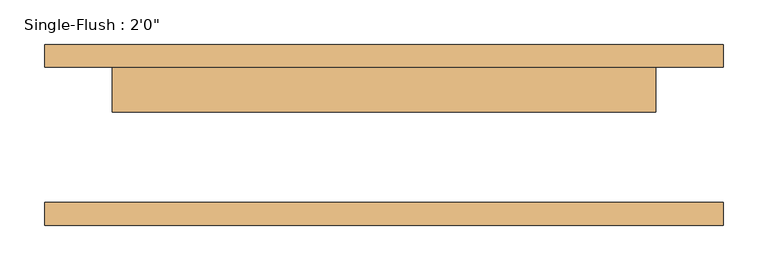
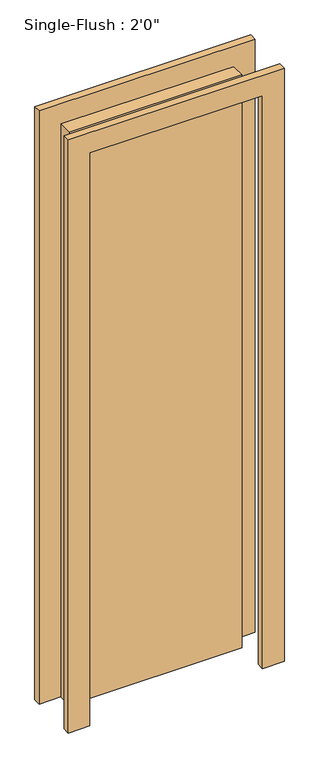
"""IFC4 building model written with IfcOpenShell, lengths in millimetres: door geometry."""

from ifc_helpers import new_model, si_unit, frame, origin, origin_with_axes, place, context, project, spatial, polyline, outline, extrude, source, transform, mapped, element, save


def door_9ea4ff49(model_context):
    return source(origin(), model_context, "Body", "SweptSolid", [
        extrude(outline(polyline([(2209.8, -381.0), (0.0, -381.0), (0.0, -304.8), (2133.6, -304.8), (2133.6, 304.8), (0.0, 304.8), (0.0, 381.0), (2209.8, 381.0), (2209.8, -381.0)])), frame((0.0, 76.2, 0.0), z_axis=(0.0, 1.0, 0.0), x_axis=(0.0, 0.0, 1.0)), (0.0, 0.0, 1.0), 25.4),
        extrude(outline(polyline([(2209.8, 381.0), (2209.8, -381.0), (0.0, -381.0), (0.0, -304.8), (2133.6, -304.8), (2133.6, 304.8), (0.0, 304.8), (0.0, 381.0), (2209.8, 381.0)])), frame((0.0, -101.6, 0.0), z_axis=(0.0, 1.0, 0.0), x_axis=(0.0, 0.0, 1.0)), (0.0, 0.0, 1.0), 25.4),
        extrude(outline(polyline([(304.8, 25.4), (-304.8, 25.4), (-304.8, 76.2), (304.8, 76.2), (304.8, 25.4)])), origin_with_axes(), (0.0, 0.0, 1.0), 2133.6),
    ])


if __name__ == "__main__":
    model = new_model("IFC4")
    model_context = context("Model", 3, world=origin())
    ifc_project = project(units=[si_unit("LENGTHUNIT", "METRE", prefix="MILLI")], contexts=[model_context])
    site = spatial("IfcSite", under=ifc_project)
    building = spatial("IfcBuilding", under=site)
    placement = place(None, origin())
    door_shape = door_9ea4ff49(model_context)
    element("IfcDoor", 1, ObjectType="Single-Flush : 2'0\"", at=placement, inside=building, context=model_context, shape_type="MappedRepresentation", body=[
        mapped(door_shape, transform((0.0, 0.0, 0.0), x_axis=(1.0, 0.0, 0.0), y_axis=(0.0, 1.0, 0.0), z_axis=(0.0, 0.0, 1.0))),
    ])
    save(model, "model.ifc")

# Revit data of these elements
# Type "Single-Flush : 2'0\""
#   Type Mark = "9"
#   Construction Type Id = "MDOOR"
#   Assembly Code = "C1020"
#   Analytic Construction = "Metal"
#   Thickness = 0' - 2"
#   Heat Transfer Coefficient (U) = 0.651978 BTU/(h·ft²·°F)
#   Height = 7' - 0"
#   Trim Projection Ext = 0' - 1"
#   Trim Projection Int = 0' - 1"
#   Trim Width = 0' - 3"
#   Width = 2' - 0"
#   Define Thermal Properties by = 1
#   Door Material = Door - Panel
#   Frame Material = Door - Frame
#   Visual Light Transmittance = 0
#   Solar Heat Gain Coefficient = 0
#   Function = (empty or 0)
#   Wall Closure = (empty or 0)
# Element 1 (IfcDoor, "Single-Flush : 2'0\"")
#   Materials on its faces: "Door - Frame", "Door - Panel"
# Materials
#   "Door - Panel": class "Wood", colour RGB 210 159 95, transparency 0, Cost = 0
#   "Door - Frame": colour RGB 118 70 51, transparency 0, Cost = 0
